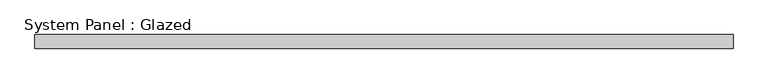
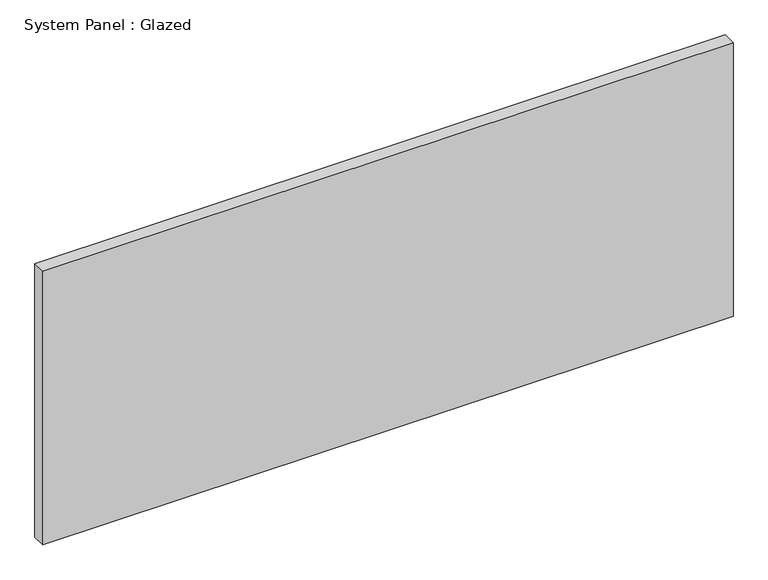
"""IFC4 building model written with IfcOpenShell, lengths in millimetres: plate geometry, System Panel : Glazed."""

from ifc_helpers import new_model, si_unit, origin, origin_with_axes, place, context, project, spatial, polyline, outline, extrude, source, transform, mapped, element, save


def system_panel_glazed_17e06366(model_context):
    return source(origin(), model_context, "Body", "SweptSolid", [
        extrude(outline(polyline([(651.4041668, 19.05), (-651.4041668, 19.05), (-651.4041668, 44.45), (651.4041668, 44.45), (651.4041668, 19.05)])), origin_with_axes(), (0.0, 0.0, 1.0), 546.1),
    ])


if __name__ == "__main__":
    model = new_model("IFC4")
    model_context = context("Model", 3, world=origin())
    ifc_project = project(units=[si_unit("LENGTHUNIT", "METRE", prefix="MILLI")], contexts=[model_context])
    site = spatial("IfcSite", under=ifc_project)
    building = spatial("IfcBuilding", under=site)
    placement = place(None, origin())
    system_panel_glazed_shape = system_panel_glazed_17e06366(model_context)
    element("IfcPlate", 1, ObjectType="System Panel : Glazed", at=placement, inside=building, context=model_context, shape_type="MappedRepresentation", body=[
        mapped(system_panel_glazed_shape, transform((0.0, 0.0, 0.0), x_axis=(1.0, 0.0, 0.0), y_axis=(0.0, 1.0, 0.0), z_axis=(0.0, 0.0, 1.0))),
    ])
    save(model, "model.ifc")

# Revit data of these elements
# Type "System Panel : Glazed"
#   Construction Type Id = "GSP4R"
#   Analytic Construction = "1/8 in Pilkington single glazing"
#   Visual Light Transmittance = 0.9
#   Solar Heat Gain Coefficient = 0.86
#   Heat Transfer Coefficient (U) = 1.18115 BTU/(h·ft²·°F)
#   Define Thermal Properties by = 1
# Element 1 (IfcPlate, "System Panel : Glazed")
#   Materials on its faces: "Glass"
# Materials
#   "Glass": class "Glass", colour RGB 0 128 192, transparency 0.75, Description = "Soda Lime Glass", Cost = 0
